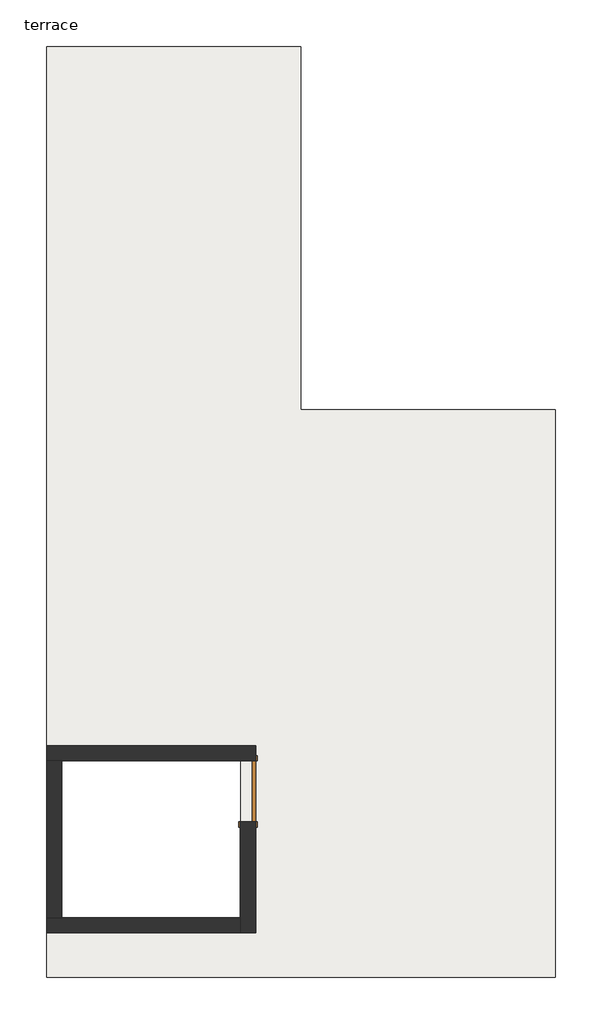
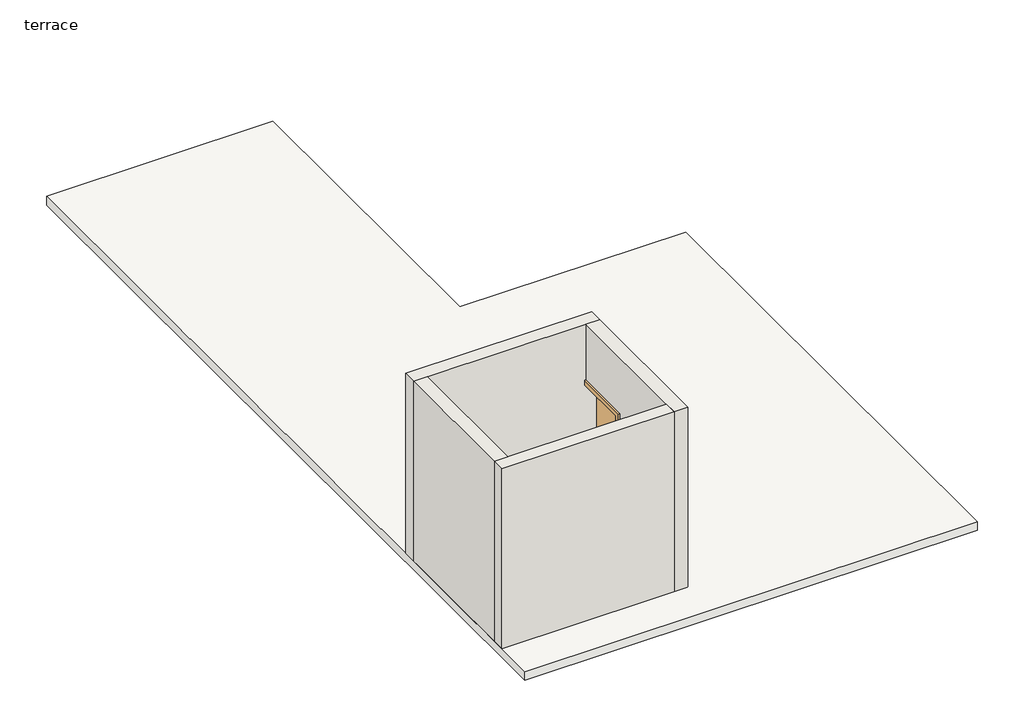
# One storey, incomplete: 4 walls, 1 door, 1 slab.
"""IFC4 building model written with IfcOpenShell, lengths in millimetres."""

from ifc_helpers import new_model, si_unit, frame, origin, place, context, project, spatial, polyline, outline, extrude, faceted_brep, transform, mapped, element, save
from components import door_0ca8825f

model = new_model("IFC4")

# Units and contexts
model_context = context("Model", 3, world=origin())
ifc_project = project(units=[si_unit("LENGTHUNIT", "METRE", prefix="MILLI")], contexts=[model_context])

# Site, building, storey
site = spatial("IfcSite", under=ifc_project)
building = spatial("IfcBuilding", under=site)
storey = spatial("IfcBuildingStorey", under=building, Name="terrace", Elevation=7010.4)

# Door
placement = place(None, origin())
door_shape = door_0ca8825f(model_context)
element("IfcDoor", 1, ObjectType="Single-Flush : 36\" x 84\"", at=placement, inside=storey, context=model_context, shape_type="MappedRepresentation", body=[
    mapped(door_shape, transform((22029.5636801, 6071.5752787, 7010.4), x_axis=(0.0, -1.0, 0.0), y_axis=(1.0, 0.0, 0.0), z_axis=(0.0, 0.0, 1.0))),
])

# Slab
element("IfcSlab", 2, at=placement, inside=storey, context=model_context, shape_type="SweptSolid", body=[
    extrude(outline(polyline([(22823.3136801, 17229.6409313), (22823.3136801, 11786.5752787), (26633.3136801, 11786.5752787), (26633.3136801, 3285.0409313), (19013.3136801, 3285.0409313), (19013.3136801, 17229.6409313), (22823.3136801, 17229.6409313)]), holes=[polyline([(19241.9136801, 6528.7752787), (19241.9136801, 4182.4502787), (21915.2636801, 4182.4502787), (21915.2636801, 5157.1752787), (21915.2636801, 6528.7752787), (19241.9136801, 6528.7752787)])]), frame((0.0, 0.0, 6858.0), z_axis=(0.0, 0.0, 1.0), x_axis=(1.0, 0.0, 0.0)), (0.0, 0.0, 1.0), 152.4),
])

# Walls
element("IfcWall", 3, at=placement, inside=storey, context=model_context, shape_type="Brep", body=[
    faceted_brep([(19013.3136801, 6528.7752787, 7010.4), (19241.9136801, 6528.7752787, 7010.4), (22143.8636801, 6528.7752787, 7010.4), (22143.8636801, 6528.7752787, 9144.0), (22143.8636801, 6528.7752787, 10210.8), (21915.2636801, 6528.7752787, 10210.8), (19241.9136801, 6528.7752787, 10210.8), (19013.3136801, 6528.7752787, 10210.8), (19013.3136801, 6757.3752787, 7010.4), (19013.3136801, 6757.3752787, 10210.8), (22143.8636801, 6757.3752787, 10210.8), (22143.8636801, 6757.3752787, 7010.4)], [[[0, 1, 2, 3, 4, 5, 6, 7]], [[8, 9, 10, 11]], [[2, 1, 0, 8, 11]], [[7, 6, 5, 4, 10, 9]], [[4, 3, 2, 11, 10]], [[0, 7, 9, 8]]]),
])
element("IfcWall", 4, at=placement, inside=storey, context=model_context, shape_type="Brep", body=[
    faceted_brep([(21915.2636801, 3953.8502787, 10210.8), (21915.2636801, 4182.4502787, 10210.8), (21915.2636801, 6528.7752787, 10210.8), (21915.2636801, 6528.7752787, 9144.0), (21915.2636801, 5614.3752787, 9144.0), (21915.2636801, 5614.3752787, 7010.4), (21915.2636801, 4182.4502787, 7010.4), (21915.2636801, 3953.8502787, 7010.4), (22143.8636801, 6528.7752787, 10210.8), (22143.8636801, 3953.8502787, 10210.8), (22143.8636801, 3953.8502787, 7010.4), (22143.8636801, 5614.3752787, 7010.4), (22143.8636801, 5614.3752787, 9144.0), (22143.8636801, 6528.7752787, 9144.0)], [[[0, 1, 2, 3, 4, 5, 6, 7]], [[8, 9, 10, 11, 12, 13]], [[10, 7, 6, 5, 11]], [[2, 1, 0, 9, 8]], [[2, 8, 13, 3]], [[0, 7, 10, 9]], [[4, 12, 11, 5]], [[12, 4, 3, 13]]]),
])
element("IfcWall", 5, at=placement, inside=storey, context=model_context, shape_type="Brep", body=[
    faceted_brep([(21915.2636801, 4182.4502787, 7010.4), (19241.9136801, 4182.4502787, 7010.4), (19013.3136801, 4182.4502787, 7010.4), (19013.3136801, 4182.4502787, 10210.8), (19241.9136801, 4182.4502787, 10210.8), (21915.2636801, 4182.4502787, 10210.8), (21915.2636801, 3953.8502787, 7010.4), (21915.2636801, 3953.8502787, 10210.8), (19013.3136801, 3953.8502787, 10210.8), (19013.3136801, 3953.8502787, 7010.4)], [[[0, 1, 2, 3, 4, 5]], [[6, 7, 8, 9]], [[2, 1, 0, 6, 9]], [[5, 4, 3, 8, 7]], [[0, 5, 7, 6]], [[3, 2, 9, 8]]]),
])
element("IfcWall", 6, at=placement, inside=storey, context=model_context, shape_type="SweptSolid", body=[
    extrude(outline(polyline([(19241.9136801, 6528.7752787), (19241.9136801, 4182.4502787), (19013.3136801, 4182.4502787), (19013.3136801, 6528.7752787), (19241.9136801, 6528.7752787)])), frame((0.0, 0.0, 7010.4), z_axis=(0.0, 0.0, 1.0), x_axis=(1.0, 0.0, 0.0)), (0.0, 0.0, 1.0), 3200.4),
])

save(model, "model.ifc")

# Revit data of these elements
# Type "Single-Flush : 36\" x 84\""
#   Type Mark = "1"
#   Construction Type Id = "MDOOR"
#   Assembly Code = "C1020"
#   Analytic Construction = "Metal"
#   Thickness = 0' - 2"
#   Heat Transfer Coefficient (U) = 0.651978 BTU/(h·ft²·°F)
#   Height = 7' - 0"
#   Trim Projection Ext = 0' - 1"
#   Trim Projection Int = 0' - 1"
#   Trim Width = 0' - 3"
#   Width = 3' - 0"
#   Define Thermal Properties by = 1
#   Define Thermal Properties by = 1
#   Door Material = Door - Panel
#   Frame Material = Door - Frame
#   Visual Light Transmittance = 0
#   Solar Heat Gain Coefficient = 0
#   Function = (empty or 0)
#   Wall Closure = (empty or 0)
# Type
#   Assembly Code = "B1010"
#   Function = 0
#   Layers, outside or top first: 0' - 6" "Concrete, Cast-in-Place gray" (function 1)
# Type
#   Assembly Code = "B2010"
#   Layers, outside or top first: 0' - 9" no material (function 1)
# Element 1 (IfcDoor, "Single-Flush : 36\" x 84\"")
#   Phase Created = New Construction
#   Materials on its faces: "Door - Frame", "Door - Panel"
# Element 2 (IfcSlab)
#   Height Offset From Level = 0' - 0"
#   Phase Created = New Construction
#   Materials on its faces: "Concrete, Cast-in-Place gray"
# Elements 3, 4, 5 (IfcWall)
#   Top Offset = 0' - 0"
#   Base Offset = 0' - 0"
#   wall height = 10' - 6"
#   Phase Created = New Construction
#   Base Constraint = terrace
#   Top Constraint = stair head room
#   Materials on its faces: "Default Wall", "Laminate, Ivory, Matte"
# Element 6 (IfcWall)
#   Top Offset = 0' - 0"
#   Base Offset = 0' - 0"
#   wall height = 10' - 6"
#   Phase Created = New Construction
#   Base Constraint = terrace
#   Top Constraint = stair head room
#   Materials on its faces: "Default Wall"
# Materials
#   "Door - Panel": class "Wood", colour RGB 210 159 95, transparency 0, Cost = 0
#   "Door - Frame": colour RGB 118 70 51, transparency 0, Cost = 0
#   "Concrete, Cast-in-Place gray": class "Concrete", colour RGB 192 192 192, transparency 0, Description = "Cast-in-place concrete", Cost = 0
#   "Default Wall": colour RGB 128 128 128, transparency 0, Cost = 0
#   "Laminate, Ivory, Matte": class "Plastic", colour RGB 247 247 239, transparency 0, Description = "Plastic Laminate - Ivory, Matte", Cost = 0
